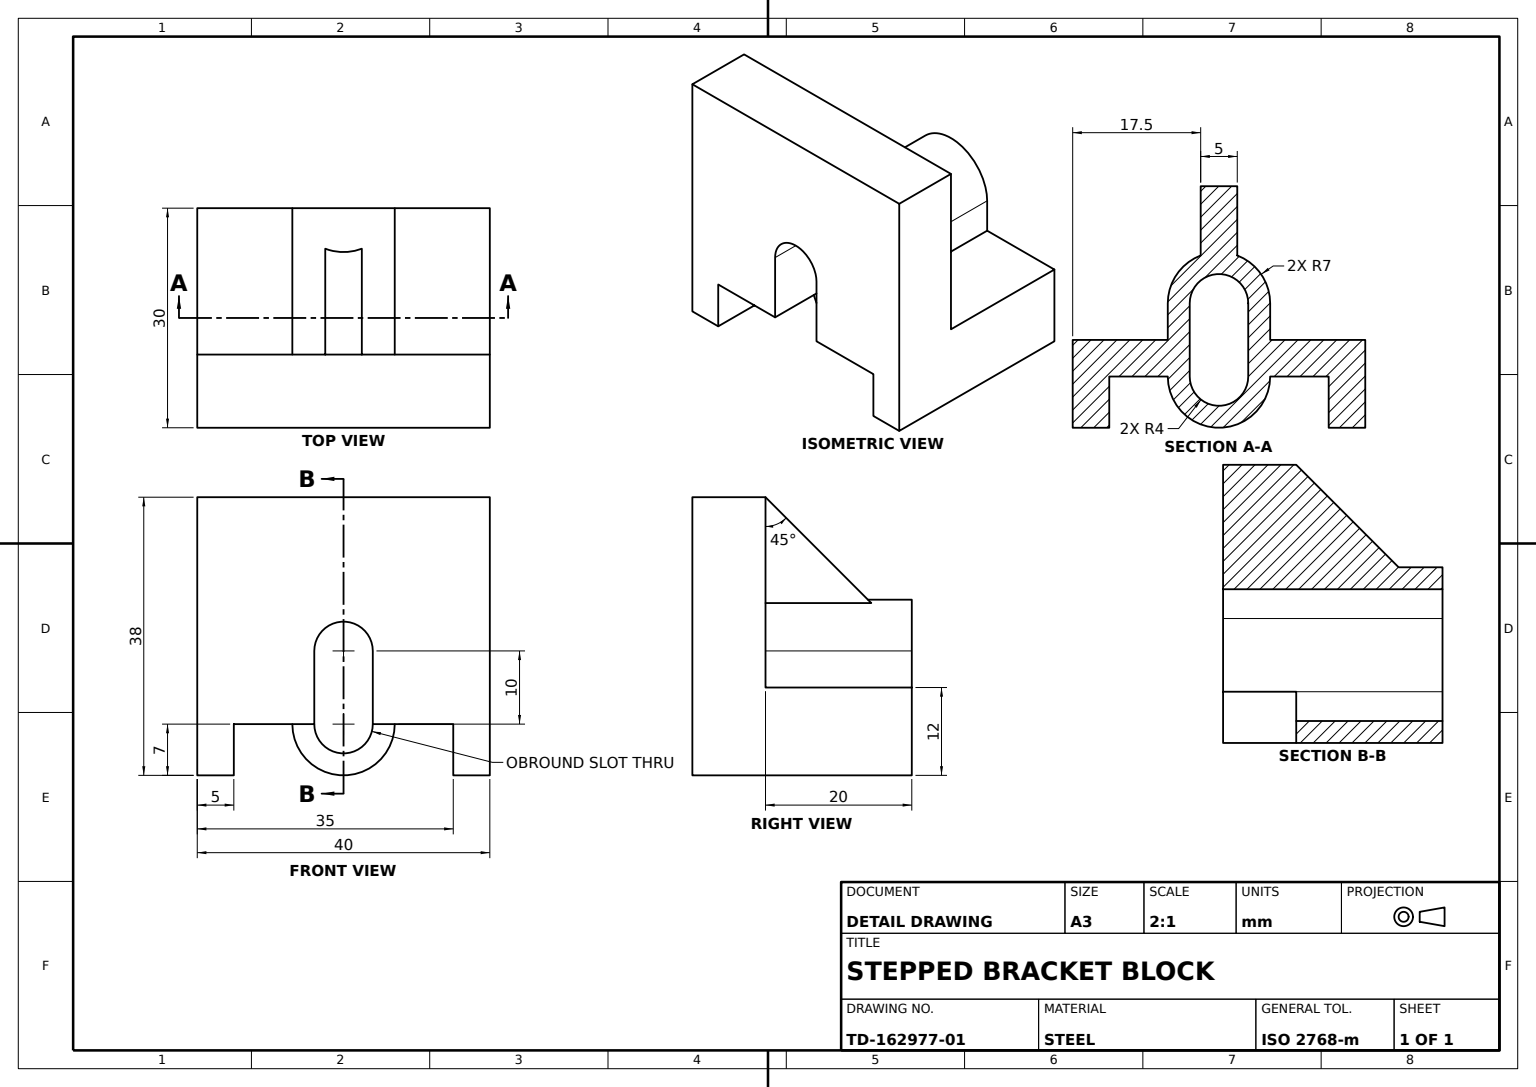
SolidWorks part; units mm, degrees
material "Plain Carbon Steel"
ref_plane "Front Plane" through (0, 0, 0) normal (0, 0, 1) x (1, 0, 0)
ref_plane "Top Plane" through (0, 0, 0) normal (0, 1, 0) x (1, 0, 0)
ref_plane "Right Plane" through (0, 0, 0) normal (1, 0, 0) x (0, 0, -1)
sketch "Bracket Profile Sketch" plane through (0, 0, 0) normal (0, 0, 1) x (1, 0, 0)
  line L0 (0, 0) -> (30, 0)
  line L1 (30, 0) -> (30, 38)
  line L2 (30, 38) -> (20, 38)
  line L3 (0, 0) -> (0, 12)
  line L4 (0, 12) -> (20, 12)
  line L5 (20, 12) -> (20, 38)
  dimension "D1" = 30
  dimension "D2" = 38
  dimension "D3" = 12
  dimension "D4" = 20
extrude "Bracket Body" add sketch "Bracket Profile Sketch" along normal blind 40
sketch "Base Notch Sketch" plane through (0, 0, 0) normal (-1, 0, 0) x (0, 0, 1)
  line L0 (0, 0) -> (5, 0)
  line L2 (40, 0) -> (0, 0) construction
  line L3 (5, 0) -> (5, 7)
  line L4 (40, 0) -> (35, 0)
  line L5 (35, 0) -> (35, 7)
  line L6 (35, 7) -> (5, 7)
  line L7 (5, 0) -> (35, 0)
  line M5 (0, 0) -> (40, 0)
  dimension "D1" = 5
  dimension "D2" = 5
  dimension "D3" = 35
  dimension "D4" = 7
extrude "Base Notch Cut" cut sketch "Base Notch Sketch" against normal through all contours L5 L6 L3 M5
sketch "Cylindrical Boss Sketch" plane through (0, 0, 0) normal (-1, 0, 0) x (0, 0, 1)
  line L0 (20, 7) -> (20, 17) construction
  line L1 (35, 7) -> (5, 7) construction
  line L2 (16, 7) -> (16, 17)
  line L3 (24, 7) -> (24, 17)
  line L4 (20, 7) -> (20, 17) construction
  line L5 (40, 12) -> (0, 12) construction
  line L6 (13, 7) -> (13, 17)
  line L7 (27, 7) -> (27, 17)
  arc A0 (16, 7) -> (24, 7) centre (20, 7) ccw
  arc A1 (24, 17) -> (16, 17) centre (20, 17) ccw
  arc A2 (13, 7) -> (27, 7) centre (20, 7) ccw
  arc A3 (27, 17) -> (13, 17) centre (20, 17) ccw
  point P4 (20, 12)
  point P13 (20, 12)
  dimension "D2" = 4
  dimension "D3" = 7
  dimension "D1" = 10
extrude "Cylindrical Boss" add sketch "Cylindrical Boss Sketch" against normal blind 20
sketch "Upright Opening Sketch" plane through (0, 0, 0) normal (-1, 0, 0) x (0, 0, 1)
  line L0 (16, 12) -> (16, 7)
  line L1 (16, 7) -> (24, 7)
  line L2 (24, 7) -> (24, 12)
  line L3 (24, 12) -> (16, 12)
  arc A0 (16, 7) -> (24, 7) centre (20, 7) ccw construction
extrude "Upright Opening Cut" cut sketch "Upright Opening Sketch" against normal blind 20
sketch "Arched Relief Sketch" plane through (20, 0, 0) normal (-1, 0, 0) x (0, 0, 1)
  line L0 (16, 17) -> (16, 7)
  line L1 (16, 7) -> (24, 7)
  line L2 (24, 7) -> (24, 17)
  line L3 (24, 7) -> (24, 17) construction
  line L4 (24, 7) -> (24, 17) construction
  arc A0 (16, 17) -> (24, 17) centre (20, 17) cw
extrude "Arched Relief Cut" cut sketch "Arched Relief Sketch" against normal through all
ref_plane "Rib Plane" through (0, 0, 20) normal (0, 0, 1) x (1, 0, 0)
sketch "Support Rib Sketch" plane through (0, 0, 20) normal (0, 0, 1) x (1, 0, 0)
  line L0 (20, 38) -> (6, 24)
  line L1 (20, 24) -> (0, 24) construction
  dimension "D1" = 45
rib "Support Rib 45deg" sketch "Support Rib Sketch" sketch "Support Rib Sketch" thickness 5 extrusion direction parallel to sketch draft on no parameters "D1"=5
